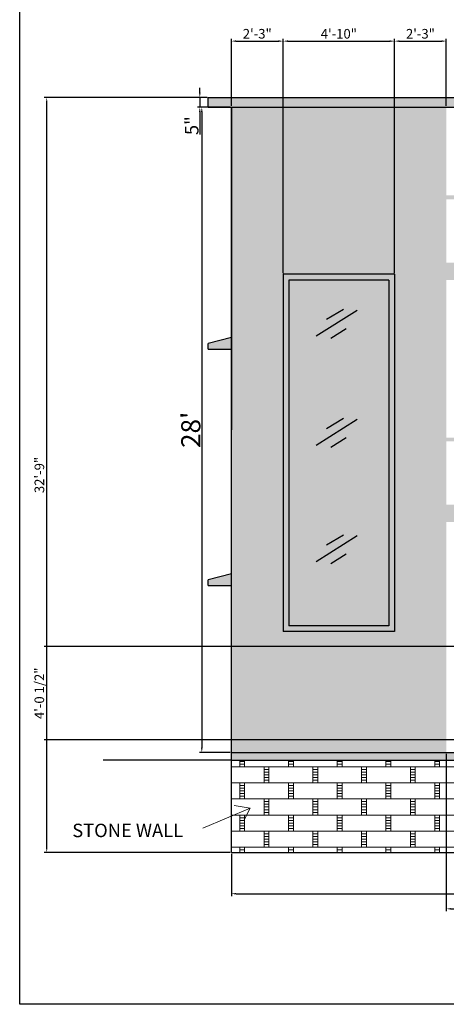
# Model space of a CAD drawing. Units: inches. Extents: x 1662 to 23131, y 1265 to 19127.
# Tile 9 of 26: x 17165 to 17387, y 7742 to 8255. Entities that reach past the tile are written whole.
import ezdxf

# ---------------------------------------------------------------- set-up
doc = ezdxf.new("R2010")
doc.units = ezdxf.units.IN
for name, color, linetype, lineweight in [('A-ANNO-DIMS', 4, 'Continuous', 18), ('A-ANNO-TEXT', 7, 'Continuous', 18), ('A-ANNO-TTLB', 7, 'Continuous', 25), ('A-ELEV', 7, 'Continuous', 25), ('A-ELEV-PATT', 8, 'Continuous', 13), ('A-ELEV-SURF-PATT', 252, 'Continuous', 13)]:
    doc.layers.add(name, color=color, linetype=linetype, lineweight=lineweight)
doc.styles.get("Standard").update_dxf_attribs({"font": 'arial.ttf'})
doc.dimstyles.new('ISO-25', dxfattribs={"dimtxt": 5, "dimasz": 2.5, "dimexe": 1.25, "dimexo": 0.625, "dimtad": 1, "dimlunit": 3, "dimtxsty": 'Standard', "dimcen": 2.5, "dimadec": 0, "dimazin": 0, "dimtfac": 1, "dimtmove": 0, "dimatfit": 3, "dimfxl": 1, "dimarcsym": 0})

# ---------------------------------------------------------------- blocks, each defined once
blk = doc.blocks.new('*D76')
at = {"layer": 'A-ANNO-DIMS', "color": 0, "lineweight": -2, "transparency": 16777216}
for p, q in [((17274.63, 8209.16), (17258.62, 8209.16)), ((17259.87, 8206.66), (17259.87, 7875.66)), ((17274.63, 7873.16), (17258.62, 7873.16))]:
    blk.add_line(p, q, dxfattribs=at)
at = {"layer": 'A-ANNO-DIMS', "color": 0, "transparency": 16777216}
for points in [[(17259.45, 8206.66), (17260.28, 8206.66), (17259.87, 8209.16)], [(17259.45, 7875.66), (17260.28, 7875.66), (17259.87, 7873.16)]]:
    blk.add_solid(points, dxfattribs=at)
at = {"layer": 'Defpoints', "color": 0, "transparency": 16777216}
for p in [(17275.26, 8209.16), (17259.87, 7873.16), (17275.26, 7873.16)]:
    blk.add_point(p, dxfattribs=at)
at = {"layer": 'A-ANNO-DIMS', "color": 0, "transparency": 16777216, "insert": (17254.14, 8041.16), "char_height": 5, "attachment_point": 5, "rotation": 90}
blk.add_mtext("{\\H2x;28'}", dxfattribs=at)
blk = doc.blocks.new('*D77')
at = {"layer": 'A-ANNO-DIMS', "color": 0, "lineweight": -2, "transparency": 16777216}
for p, q in [((17258.83, 8216.66), (17258.83, 8219.16)), ((17262.63, 8214.16), (17257.58, 8214.16)), ((17258.83, 8214.16), (17258.83, 8209.16)), ((17262.63, 8209.16), (17257.58, 8209.16)), ((17258.83, 8206.66), (17258.83, 8194.86))]:
    blk.add_line(p, q, dxfattribs=at)
at = {"layer": 'A-ANNO-DIMS', "color": 0, "transparency": 16777216}
for points in [[(17258.41, 8216.66), (17259.24, 8216.66), (17258.83, 8214.16)], [(17258.41, 8206.66), (17259.24, 8206.66), (17258.83, 8209.16)]]:
    blk.add_solid(points, dxfattribs=at)
at = {"layer": 'Defpoints', "color": 0, "transparency": 16777216}
for p in [(17263.26, 8214.16), (17258.83, 8209.16), (17263.26, 8209.16)]:
    blk.add_point(p, dxfattribs=at)
at = {"layer": 'A-ANNO-DIMS', "color": 0, "transparency": 16777216, "insert": (17254.64, 8199.51), "char_height": 5, "attachment_point": 5, "rotation": 90}
blk.add_mtext('{\\H1.4x;5"}', dxfattribs=at)
blk = doc.blocks.new('*D85')
at = {"layer": 'A-ANNO-DIMS', "color": 0, "lineweight": -2, "transparency": 16777216}
for p, q in [((17275.26, 7820.53), (17275.26, 7798.45)), ((17693.26, 7820.53), (17693.26, 7798.45)), ((17277.76, 7799.7), (17690.76, 7799.7))]:
    blk.add_line(p, q, dxfattribs=at)
at = {"layer": 'A-ANNO-DIMS', "color": 0, "transparency": 16777216}
for points in [[(17277.76, 7800.12), (17277.76, 7799.28), (17275.26, 7799.7)], [(17690.76, 7800.12), (17690.76, 7799.28), (17693.26, 7799.7)]]:
    blk.add_solid(points, dxfattribs=at)
at = {"layer": 'Defpoints', "color": 0, "transparency": 16777216}
for p in [(17275.26, 7821.16), (17693.26, 7821.16), (17693.26, 7799.7)]:
    blk.add_point(p, dxfattribs=at)
at = {"layer": 'A-ANNO-DIMS', "color": 0, "transparency": 16777216, "insert": (17484.26, 7805.43), "char_height": 5, "attachment_point": 5}
blk.add_mtext('{\\H2x;34\'-10"}', dxfattribs=at)
blk = doc.blocks.new('*D230')
at = {"layer": 'A-ANNO-DIMS', "color": 0, "lineweight": -2, "transparency": 16777216}
for p, q in [((17262.63, 8214.16), (17177.82, 8214.16)), ((17179.07, 7823.66), (17179.07, 8211.66)), ((17274.63, 7821.16), (17177.82, 7821.16))]:
    blk.add_line(p, q, dxfattribs=at)
at = {"layer": 'A-ANNO-DIMS', "color": 0, "transparency": 16777216}
for points in [[(17178.65, 8211.66), (17179.48, 8211.66), (17179.07, 8214.16)], [(17178.65, 7823.66), (17179.48, 7823.66), (17179.07, 7821.16)]]:
    blk.add_solid(points, dxfattribs=at)
at = {"layer": 'Defpoints', "color": 0, "transparency": 16777216}
for p in [(17179.07, 8214.16), (17263.26, 8214.16), (17275.26, 7821.16)]:
    blk.add_point(p, dxfattribs=at)
at = {"layer": 'A-ANNO-DIMS', "color": 0, "transparency": 16777216, "insert": (17175.89, 8017.66), "char_height": 5, "attachment_point": 5, "rotation": 90}
blk.add_mtext('32\'-9"', dxfattribs=at)
blk = doc.blocks.new('*D231')
at = {"layer": 'A-ANNO-DIMS', "color": 0, "lineweight": -2, "transparency": 16777216}
for p, q in [((17275.26, 8209.78), (17275.26, 8244.76)), ((17277.76, 8243.51), (17299.76, 8243.51)), ((17302.26, 8122.78), (17302.26, 8244.76))]:
    blk.add_line(p, q, dxfattribs=at)
at = {"layer": 'A-ANNO-DIMS', "color": 0, "transparency": 16777216}
for points in [[(17277.76, 8243.93), (17277.76, 8243.09), (17275.26, 8243.51)], [(17299.76, 8243.93), (17299.76, 8243.09), (17302.26, 8243.51)]]:
    blk.add_solid(points, dxfattribs=at)
at = {"layer": 'Defpoints', "color": 0, "transparency": 16777216}
for p in [(17302.26, 8243.51), (17275.26, 8209.16), (17302.26, 8122.16)]:
    blk.add_point(p, dxfattribs=at)
at = {"layer": 'A-ANNO-DIMS', "color": 0, "transparency": 16777216, "insert": (17288.76, 8246.69), "char_height": 5, "attachment_point": 5}
blk.add_mtext('2\'-3"', dxfattribs=at)
blk = doc.blocks.new('*D232')
at = {"layer": 'A-ANNO-DIMS', "color": 0, "lineweight": -2, "transparency": 16777216}
for p, q in [((17302.26, 8122.78), (17302.26, 8244.76)), ((17304.76, 8243.51), (17357.76, 8243.51)), ((17360.26, 8122.78), (17360.26, 8244.76))]:
    blk.add_line(p, q, dxfattribs=at)
at = {"layer": 'A-ANNO-DIMS', "color": 0, "transparency": 16777216}
for points in [[(17304.76, 8243.93), (17304.76, 8243.09), (17302.26, 8243.51)], [(17357.76, 8243.93), (17357.76, 8243.09), (17360.26, 8243.51)]]:
    blk.add_solid(points, dxfattribs=at)
at = {"layer": 'Defpoints', "color": 0, "transparency": 16777216}
for p in [(17360.26, 8243.51), (17302.26, 8122.16), (17360.26, 8122.16)]:
    blk.add_point(p, dxfattribs=at)
at = {"layer": 'A-ANNO-DIMS', "color": 0, "transparency": 16777216, "insert": (17331.26, 8246.69), "char_height": 5, "attachment_point": 5}
blk.add_mtext('4\'-10"', dxfattribs=at)
blk = doc.blocks.new('*D233')
at = {"layer": 'A-ANNO-DIMS', "color": 0, "lineweight": -2, "transparency": 16777216}
for p, q in [((17360.26, 8122.78), (17360.26, 8244.76)), ((17362.76, 8243.51), (17384.76, 8243.51)), ((17387.26, 8209.78), (17387.26, 8244.76))]:
    blk.add_line(p, q, dxfattribs=at)
at = {"layer": 'A-ANNO-DIMS', "color": 0, "transparency": 16777216}
for points in [[(17362.76, 8243.93), (17362.76, 8243.09), (17360.26, 8243.51)], [(17384.76, 8243.93), (17384.76, 8243.09), (17387.26, 8243.51)]]:
    blk.add_solid(points, dxfattribs=at)
at = {"layer": 'Defpoints', "color": 0, "transparency": 16777216}
for p in [(17387.26, 8243.51), (17387.26, 8209.16), (17360.26, 8122.16)]:
    blk.add_point(p, dxfattribs=at)
at = {"layer": 'A-ANNO-DIMS', "color": 0, "transparency": 16777216, "insert": (17373.76, 8246.69), "char_height": 5, "attachment_point": 5}
blk.add_mtext('2\'-3"', dxfattribs=at)
blk = doc.blocks.new('*D237')
at = {"layer": 'A-ANNO-DIMS', "color": 0, "lineweight": -2, "transparency": 16777216}
for p, q in [((17387.26, 7872.53), (17387.26, 7790.56)), ((17585.26, 7872.53), (17585.26, 7790.56)), ((17389.76, 7791.81), (17582.76, 7791.81))]:
    blk.add_line(p, q, dxfattribs=at)
at = {"layer": 'A-ANNO-DIMS', "color": 0, "transparency": 16777216}
for points in [[(17389.76, 7792.23), (17389.76, 7791.39), (17387.26, 7791.81)], [(17582.76, 7792.23), (17582.76, 7791.39), (17585.26, 7791.81)]]:
    blk.add_solid(points, dxfattribs=at)
at = {"layer": 'Defpoints', "color": 0, "transparency": 16777216}
for p in [(17387.26, 7873.16), (17585.26, 7873.16), (17585.26, 7791.81)]:
    blk.add_point(p, dxfattribs=at)
at = {"layer": 'A-ANNO-DIMS', "color": 0, "transparency": 16777216, "insert": (17486.26, 7794.99), "char_height": 5, "attachment_point": 5}
blk.add_mtext('16\'-6"', dxfattribs=at)
blk = doc.blocks.new('*D240')
at = {"layer": 'A-ANNO-DIMS', "color": 0, "lineweight": -2, "transparency": 16777216}
for p, q in [((17399.43, 7928.32), (17177.82, 7928.32)), ((17179.07, 7882.22), (17179.07, 7925.82)), ((17399.43, 7879.72), (17177.82, 7879.72))]:
    blk.add_line(p, q, dxfattribs=at)
at = {"layer": 'A-ANNO-DIMS', "color": 0, "transparency": 16777216}
for points in [[(17178.65, 7925.82), (17179.48, 7925.82), (17179.07, 7928.32)], [(17178.65, 7882.22), (17179.48, 7882.22), (17179.07, 7879.72)]]:
    blk.add_solid(points, dxfattribs=at)
at = {"layer": 'Defpoints', "color": 0, "transparency": 16777216}
for p in [(17179.07, 7928.32), (17400.05, 7928.32), (17400.05, 7879.72)]:
    blk.add_point(p, dxfattribs=at)
at = {"layer": 'A-ANNO-DIMS', "color": 0, "transparency": 16777216, "insert": (17175.86, 7904.02), "char_height": 5, "attachment_point": 5, "rotation": 90}
blk.add_mtext('4\'-0 1/2"', dxfattribs=at)

msp = doc.modelspace()

# ---------------------------------------------------------------- hatches: boundary and pattern name
at = {"layer": 'A-ELEV-PATT'}
h = msp.add_hatch(dxfattribs=at)
h.set_pattern_fill('BRSTONE', color=256)
h.set_pattern_definition([(0, (0, 78.8975), (0, 8.382), []), (90, (22.86, 78.898), (-12.7, 8.382), [8.382, -8.382]), (90, (20.32, 78.898), (-12.7, 8.382), [8.382, -8.382]), (0, (22.86, 80.2945), (12.7, 8.382), [-22.86, 2.54]), (0, (22.86, 81.6915), (12.7, 8.382), [-22.86, 2.54]), (0, (22.86, 83.0885), (12.7, 8.382), [-22.86, 2.54]), (0, (22.86, 84.4855), (12.7, 8.382), [-22.86, 2.54]), (0, (22.86, 85.8825), (12.7, 8.382), [-22.86, 2.54])])
h.paths.add_polyline_path([(17693.258, 7821.159), (17693.258, 7869.159), (17275.258, 7869.159), (17275.258, 7821.159)])
at = {"layer": 'A-ELEV-SURF-PATT'}
h = msp.add_hatch(color=256, dxfattribs=at)
h.dxf.hatch_style = 1
h.paths.add_polyline_path([(17263.258, 8214.159), (17263.258, 8209.159), (17411.258, 8209.159), (17411.258, 8214.159)])
h.paths.add_polyline_path([(17699.258, 8119.159), (17699.258, 8125.159), (17693.258, 8125.159), (17693.258, 8128.159), (17684.258, 8128.159), (17616.758, 8128.159), (17607.758, 8128.159), (17544.758, 8128.159), (17535.758, 8128.159), (17472.758, 8128.159), (17463.758, 8128.159), (17396.258, 8128.159), (17387.258, 8128.159), (17387.258, 8119.159)])
h.paths.add_polyline_path([(17699.258, 7993.159), (17699.258, 7999.159), (17693.258, 7999.159), (17693.258, 8002.159), (17684.258, 8002.159), (17616.758, 8002.159), (17607.758, 8002.159), (17544.758, 8002.159), (17535.758, 8002.159), (17472.758, 8002.159), (17463.758, 8002.159), (17396.258, 8002.159), (17387.258, 8002.159), (17387.258, 7993.159)])
h.paths.add_polyline_path([(17693.258, 7869.159), (17693.258, 7873.159), (17275.258, 7873.159), (17275.258, 7869.159)])
h.paths.add_polyline_path([(17396.258, 8035.159), (17398.258, 8035.159), (17398.258, 8037.159), (17396.258, 8037.159), (17387.258, 8037.159), (17387.258, 8035.159)])
h.paths.add_polyline_path([(17473.258, 8035.159), (17474.758, 8035.159), (17474.758, 8037.159), (17461.758, 8037.159), (17461.758, 8035.159)])
h.paths.add_polyline_path([(17546.758, 8037.159), (17544.758, 8037.159), (17535.758, 8037.159), (17533.758, 8037.159), (17533.758, 8035.159), (17535.758, 8035.159), (17544.758, 8035.159), (17546.758, 8035.159)])
h.paths.add_polyline_path([(17616.758, 8035.159), (17618.758, 8035.159), (17618.758, 8037.159), (17616.758, 8037.159), (17607.758, 8037.159), (17605.758, 8037.159), (17605.758, 8035.159), (17607.758, 8035.159)])
h.paths.add_polyline_path([(17695.258, 8035.159), (17695.258, 8037.159), (17684.258, 8037.159), (17682.258, 8037.159), (17682.258, 8035.159), (17684.258, 8035.159)])
h.paths.add_polyline_path([(17684.258, 8163.159), (17682.258, 8163.159), (17682.258, 8161.159), (17684.258, 8161.159), (17693.258, 8161.159), (17695.258, 8161.159), (17695.258, 8163.159), (17693.258, 8163.159)])
h.paths.add_polyline_path([(17616.758, 8161.159), (17618.758, 8161.159), (17618.758, 8163.159), (17616.758, 8163.159), (17607.758, 8163.159), (17605.758, 8163.159), (17605.758, 8161.159), (17607.758, 8161.159)])
h.paths.add_polyline_path([(17544.758, 8161.159), (17546.758, 8161.159), (17546.758, 8163.159), (17544.758, 8163.159), (17535.758, 8163.159), (17533.758, 8163.159), (17533.758, 8161.159), (17535.758, 8161.159)])
h.paths.add_polyline_path([(17463.758, 8163.159), (17461.758, 8163.159), (17461.758, 8161.159), (17463.758, 8161.159), (17472.758, 8161.159), (17474.758, 8161.159), (17474.758, 8163.159), (17472.758, 8163.159)])
h.paths.add_polyline_path([(17396.258, 8161.159), (17398.258, 8161.159), (17398.258, 8163.159), (17396.258, 8163.159), (17387.258, 8163.159), (17387.258, 8161.159)])
h.paths.add_polyline_path([(17711.258, 8083.159), (17711.258, 8086.159), (17693.258, 8089.159), (17693.258, 8083.159)])
h.paths.add_polyline_path([(17711.258, 7960.159), (17711.258, 7963.159), (17693.258, 7966.159), (17693.258, 7960.159)])
h.paths.add_polyline_path([(17263.258, 7963.159), (17263.258, 7960.159), (17275.258, 7960.159), (17275.258, 7966.159)])
h.paths.add_polyline_path([(17275.258, 8083.159), (17275.258, 8089.159), (17263.258, 8086.159), (17263.258, 8083.159)])
h = msp.add_hatch(color=256, dxfattribs=at)
h.dxf.hatch_style = 1
h.paths.add_polyline_path([(17275.258, 8209.159), (17275.258, 8041.159), (17275.258, 7873.159), (17387.258, 7873.159), (17387.258, 8209.159)])
h.paths.add_polyline_path([(17360.258, 8122.159), (17360.258, 7936.159), (17302.258, 7936.159), (17302.258, 8122.159)], flags=16)
h.paths.add_polyline_path([(17357.258, 8119.159), (17357.258, 7939.159), (17305.258, 7939.159), (17305.258, 8119.159)], flags=0)
h = msp.add_hatch(color=256, dxfattribs=at)
h.dxf.hatch_style = 1
h.paths.add_polyline_path([(17360.258, 7936.159), (17360.258, 8122.159), (17302.258, 8122.159), (17302.258, 7936.159)])
h.paths.add_polyline_path([(17305.258, 7939.159), (17305.258, 8119.159), (17357.258, 8119.159), (17357.258, 7939.159)], flags=16)
h = msp.add_hatch(color=256, dxfattribs=at)
h.dxf.hatch_style = 1
h.paths.add_polyline_path([(17302.258, 7936.159), (17360.258, 7936.159), (17360.258, 8122.159), (17302.258, 8122.159)])
h.paths.add_polyline_path([(17305.258, 8119.159), (17357.258, 8119.159), (17357.258, 7939.159), (17305.258, 7939.159)], flags=16)
h = msp.add_hatch(color=256, dxfattribs=at)
h.dxf.hatch_style = 1
h.paths.add_polyline_path([(17357.258, 8119.159), (17305.258, 8119.159), (17305.258, 7939.159), (17357.258, 7939.159)])

# ---------------------------------------------------------------- linework, layer by layer
at = {"layer": 'A-ANNO-TEXT'}
for p, q in [((17260.48, 7833.725), (17284.979, 7844.212)), ((17284.979, 7844.212), (17276.654, 7845.537)), ((17284.979, 7844.212), (17281.748, 7837.759)), ((17284.979, 7844.212), (17284.979, 7844.212))]:
    msp.add_line(p, q, dxfattribs=at)
at = {"layer": 'A-ANNO-TTLB'}
msp.add_lwpolyline([(17164.976, 8731.935), (18265.142, 8731.935), (18265.142, 7742.121), (17164.976, 7742.121)], close=True, dxfattribs=at)
at = {"layer": 'A-ELEV'}
for p, q in [((17263.258, 8214.159), (17411.258, 8214.159)), ((17263.258, 8209.159), (17263.258, 8214.159)), ((17263.258, 8209.159), (17411.258, 8209.159)), ((17275.258, 7821.159), (17275.258, 8209.159)), ((17275.258, 8209.159), (17275.258, 8041.159)), ((17360.258, 8122.159), (17302.258, 8122.159)), ((17302.258, 8122.159), (17302.258, 7936.159)), ((17357.258, 8119.159), (17305.258, 8119.159)), ((17305.258, 8119.159), (17305.258, 7939.159)), ((17357.258, 8119.159), (17357.258, 7939.159)), ((17360.258, 8122.159), (17360.258, 7936.159)), ((17319.45, 8090.024), (17340.779, 8103.503)), ((17324.875, 8098.697), (17333.766, 8103.94)), ((17327.125, 8088.96), (17335.159, 8093.989)), ((17275.258, 8089.159), (17263.258, 8086.159)), ((17263.258, 8083.159), (17263.258, 8086.159)), ((17263.258, 8083.159), (17275.258, 8083.159)), ((17324.875, 8041.932), (17333.766, 8047.175)), ((17319.45, 8033.26), (17340.779, 8046.738)), ((17327.125, 8032.196), (17335.159, 8037.224)), ((17319.45, 7972.652), (17340.779, 7986.13)), ((17324.875, 7981.324), (17333.766, 7986.567)), ((17327.125, 7971.587), (17335.159, 7976.616)), ((17275.258, 7966.159), (17263.258, 7963.159)), ((17263.258, 7960.159), (17263.258, 7963.159)), ((17263.258, 7960.159), (17275.258, 7960.159)), ((17360.258, 7936.159), (17302.258, 7936.159)), ((17357.258, 7939.159), (17305.258, 7939.159)), ((17275.258, 7873.159), (17693.258, 7873.159)), ((17275.258, 7869.159), (17208.416, 7869.159)), ((17275.258, 7869.159), (17693.258, 7869.159)), ((17275.258, 7821.159), (17693.258, 7821.159))]:
    msp.add_line(p, q, dxfattribs=at)

# ---------------------------------------------------------------- texts
at = {"layer": 'A-ANNO-TEXT', "insert": (17192.367, 7836.128), "char_height": 7, "attachment_point": 1}
msp.add_mtext_dynamic_manual_height_columns('STONE WALL', width=1142.59551, gutter_width=12.5, heights=[0], dxfattribs=at)

# ---------------------------------------------------------------- dimensions: what is measured, and where the dimension line sits
at = {"layer": 'A-ANNO-DIMS'}
for base, p1, p2, picture, middle in [((17302.258, 8243.509), (17275.258, 8209.159), (17302.258, 8122.159), '*D231', (17288.758, 8246.689)), ((17360.258, 8243.509), (17302.258, 8122.159), (17360.258, 8122.159), '*D232', (17331.258, 8246.687)), ((17387.258, 8243.509), (17360.258, 8122.159), (17387.258, 8209.159), '*D233', (17373.758, 8246.689)), ((17585.258, 7791.809), (17387.258, 7873.159), (17585.258, 7873.159), '*D237', (17486.258, 7794.987))]:
    dim = msp.add_linear_dim(base=base, p1=p1, p2=p2, dimstyle='ISO-25', override={"dimdec": 1, "dimlfac": 1, "dimrnd": 0, "dimzin": 1, "dimdsep": 46, "dimlunit": 4, "dimfrac": 2}, dxfattribs=at)
    dim.commit()
    dim.dimension.update_dxf_attribs({"geometry": picture, "text_midpoint": middle})
for base, p1, p2, text, picture, middle in [((17258.828, 8209.159), (17263.258, 8214.159), (17263.258, 8209.159), '{\\H1.4x;<>}', '*D77', (17254.643, 8199.511)), ((17259.867, 7873.159), (17275.258, 8209.159), (17275.258, 7873.159), '{\\H2x;<>}', '*D76', (17254.136, 8041.159))]:
    dim = msp.add_linear_dim(base=base, p1=p1, p2=p2, angle=90, text=text, dimstyle='ISO-25', override={"dimclrd": 0, "dimclre": 0, "dimclrt": 0}, dxfattribs=at)
    dim.commit()
    dim.dimension.update_dxf_attribs({"geometry": picture, "text_midpoint": middle})
for base, p1, p2, picture, middle in [((17179.066, 8214.159), (17275.258, 7821.159), (17263.258, 8214.159), '*D230', (17175.887, 8017.659)), ((17179.066, 7928.315), (17400.054, 7879.721), (17400.054, 7928.315), '*D240', (17175.856, 7904.018))]:
    dim = msp.add_linear_dim(base=base, p1=p1, p2=p2, angle=90, dimstyle='ISO-25', override={"dimdec": 1, "dimlfac": 1, "dimrnd": 0, "dimzin": 1, "dimdsep": 46, "dimlunit": 4, "dimfrac": 2}, dxfattribs=at)
    dim.commit()
    dim.dimension.update_dxf_attribs({"geometry": picture, "text_midpoint": middle})
dim = msp.add_linear_dim(base=(17693.258, 7799.701), p1=(17275.258, 7821.159), p2=(17693.258, 7821.159), text='{\\H2x;<>}', dimstyle='ISO-25', override={"dimclrd": 0, "dimclre": 0, "dimclrt": 0}, dxfattribs=at)
dim.commit()
dim.dimension.update_dxf_attribs({"geometry": '*D85', "text_midpoint": (17484.258, 7805.435)})

doc.saveas('drawing.dxf')
